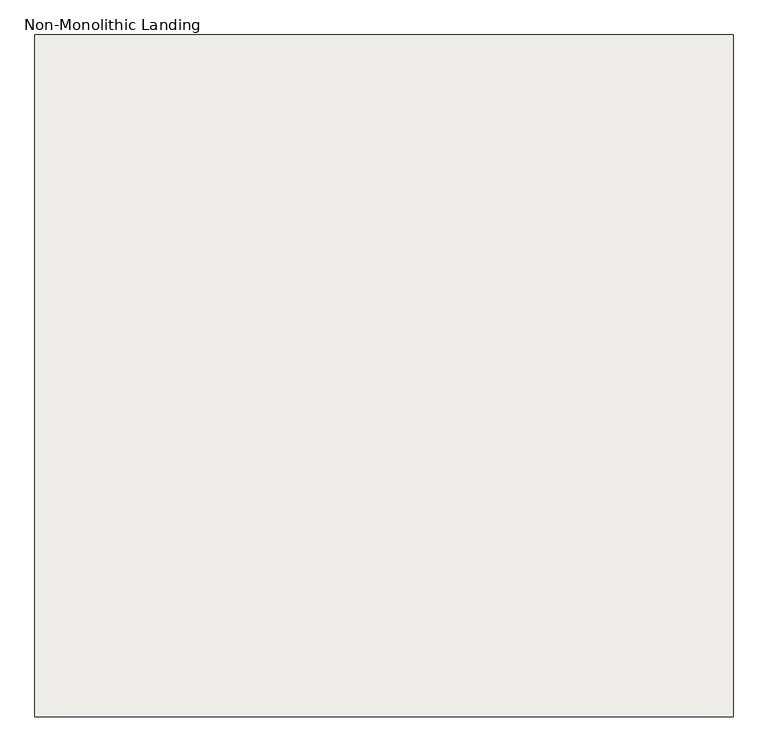
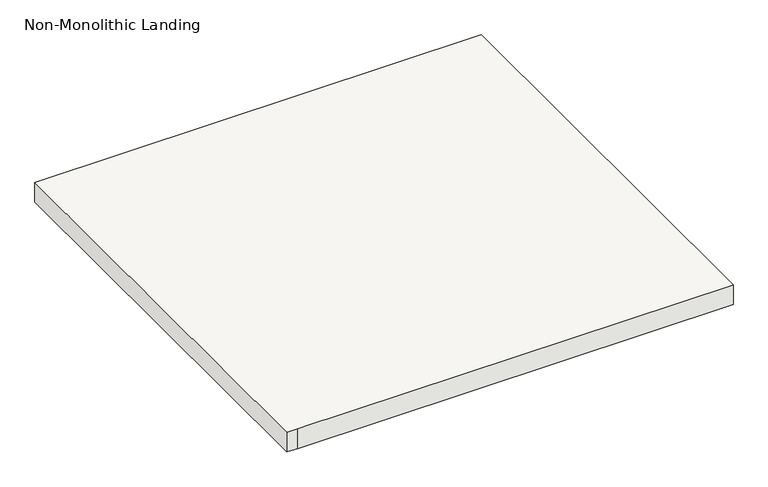
"""IFC4 building model written with IfcOpenShell, lengths in millimetres: slab geometry, Non-Monolithic Landing."""

from ifc_helpers import new_model, si_unit, origin, place, context, project, spatial, faceted_brep, source, transform, mapped, element, save


def non_monolithic_landing_665b62c1(model_context):
    return source(origin(), model_context, "Body", "Brep", [
        faceted_brep([(18745.5916032, 2869.1241878, 2609.85), (18745.5916032, 2843.7241878, 2584.45), (17678.7916032, 2843.7241878, 2584.45), (17678.7916032, 2869.1241878, 2609.85), (17653.3916032, 2869.1241878, 2628.9), (17653.3916032, 1802.3241878, 2628.9), (17678.7916032, 1802.3241878, 2628.9), (18745.5916032, 1802.3241878, 2628.9), (18745.5916032, 2869.1241878, 2628.9), (17678.7916032, 2843.7241878, 2578.1), (18745.5916032, 2843.7241878, 2578.1), (18745.5916032, 1802.3241878, 2578.1), (17678.7916032, 1802.3241878, 2578.1), (17653.3916032, 1802.3241878, 2578.1), (17653.3916032, 2869.1241878, 2578.1), (17678.7916032, 2869.1241878, 2578.1)], [[[0, 1, 2, 3]], [[4, 5, 6, 7, 8]], [[9, 10, 11, 12, 13, 14, 15]], [[10, 9, 2, 1]], [[9, 15, 3, 2]], [[4, 8, 0, 3, 15, 14]], [[5, 4, 14, 13]], [[6, 5, 13, 12]], [[7, 6, 12, 11]], [[8, 7, 11, 10, 1, 0]]]),
    ])


if __name__ == "__main__":
    model = new_model("IFC4")
    model_context = context("Model", 3, world=origin())
    ifc_project = project(units=[si_unit("LENGTHUNIT", "METRE", prefix="MILLI")], contexts=[model_context])
    site = spatial("IfcSite", under=ifc_project)
    building = spatial("IfcBuilding", under=site)
    placement = place(None, origin())
    non_monolithic_landing_shape = non_monolithic_landing_665b62c1(model_context)
    element("IfcSlab", 1, ObjectType="Non-Monolithic Landing", at=placement, inside=building, context=model_context, shape_type="MappedRepresentation", body=[
        mapped(non_monolithic_landing_shape, transform((0.0, 0.0, 0.0), x_axis=(1.0, 0.0, 0.0), y_axis=(0.0, 1.0, 0.0), z_axis=(0.0, 0.0, 1.0))),
    ])
    save(model, "model.ifc")
